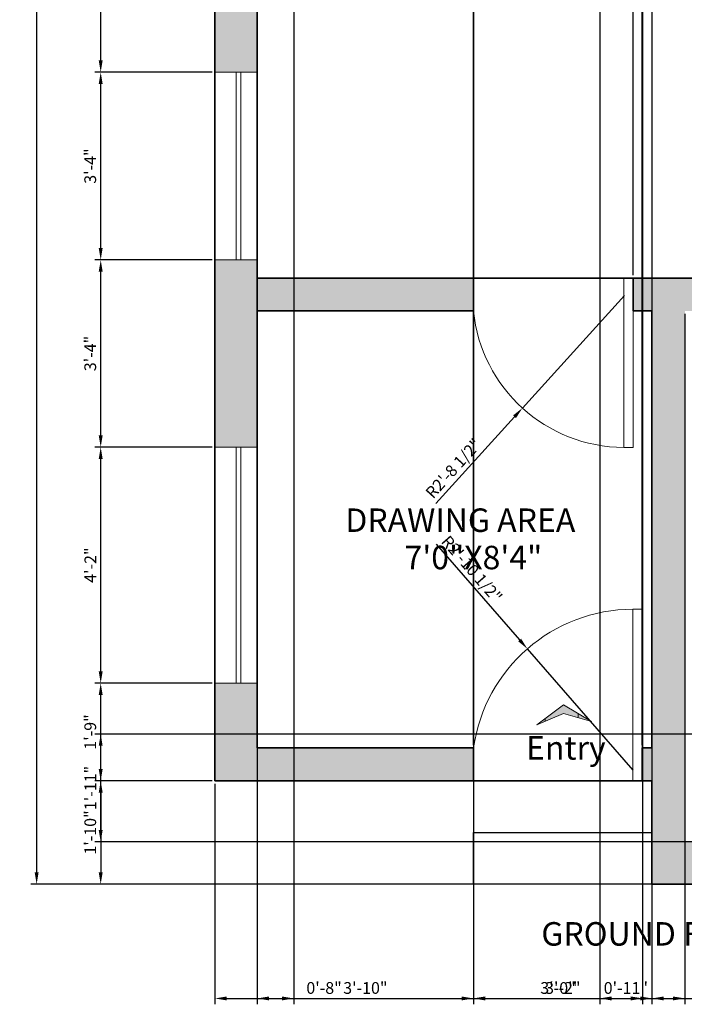
# Model space of a CAD drawing. Units: millimetres. Extents: x 2466 to 2817, y 2000 to 2512.
# Tile 1 of 4: x 2466 to 2607, y 2001 to 2210. Entities that reach past the tile are written whole.
import ezdxf

# ---------------------------------------------------------------- set-up
doc = ezdxf.new("R2010")
doc.units = ezdxf.units.MM
for name, color, linetype, lineweight in [('A-ANNO-DIMS', 2, 'Continuous', 13), ('A-ANNO-PATT', 7, 'Continuous', 13), ('A-ANNO-SYMB', 1, 'Continuous', 18), ('A-ANNO-TEXT', 7, 'Continuous', 18), ('A-AREA-IDEN', 7, 'Continuous', 18), ('A-DOOR', 3, 'Continuous', 18), ('A-FLOR-STRS', 7, 'Continuous', 25), ('A-GLAZ', 5, 'Continuous', 18), ('A-WALL', 7, 'Continuous', 35), ('A-WALL-PATT', 8, 'Continuous', 13)]:
    doc.layers.add(name, color=color, linetype=linetype, lineweight=lineweight)
doc.styles.get("Standard").update_dxf_attribs({"font": 'arial.ttf'})
doc.dimstyles.new('ISO-25', dxfattribs={"dimtxt": 2.5, "dimasz": 2.5, "dimexe": 1.25, "dimexo": 0.625, "dimtad": 1, "dimdec": 0, "dimlunit": 3, "dimtxsty": 'Standard', "dimcen": 2.5, "dimadec": 0, "dimazin": 0, "dimtfac": 1, "dimtdec": 0, "dimtmove": 0, "dimatfit": 3, "dimfxl": 1, "dimarcsym": 0})

# ---------------------------------------------------------------- blocks, each defined once
blk = doc.blocks.new('*D10')
at = {"layer": 'A-ANNO-DIMS', "color": 0, "lineweight": -2, "transparency": 16777216}
for p, q in [((2746.56, 2482.15), (2467.98, 2482.15)), ((2469.23, 2479.65), (2469.23, 2028.65)), ((2746.56, 2026.15), (2467.98, 2026.15))]:
    blk.add_line(p, q, dxfattribs=at)
at = {"layer": 'A-ANNO-DIMS', "color": 0, "transparency": 16777216}
for points in [[(2468.82, 2479.65), (2469.65, 2479.65), (2469.23, 2482.15)], [(2468.82, 2028.65), (2469.65, 2028.65), (2469.23, 2026.15)]]:
    blk.add_solid(points, dxfattribs=at)
at = {"layer": 'Defpoints', "color": 0, "transparency": 16777216}
for p in [(2747.19, 2482.15), (2469.23, 2026.15), (2747.19, 2026.15)]:
    blk.add_point(p, dxfattribs=at)
at = {"layer": 'A-ANNO-DIMS', "color": 0, "transparency": 16777216, "insert": (2467.33, 2254.15), "char_height": 2.5, "attachment_point": 5, "rotation": 90}
blk.add_mtext("38'", dxfattribs=at)
blk = doc.blocks.new('*D26')
at = {"layer": 'A-ANNO-DIMS', "color": 0, "lineweight": -2, "transparency": 16777216}
for p, q in [((2791.19, 2202.52), (2791.19, 2000.58)), ((2507.19, 2047.52), (2507.19, 2000.58)), ((2509.69, 2001.83), (2788.69, 2001.83))]:
    blk.add_line(p, q, dxfattribs=at)
at = {"layer": 'A-ANNO-DIMS', "color": 0, "transparency": 16777216}
for points in [[(2509.69, 2002.24), (2509.69, 2001.41), (2507.19, 2001.83)], [(2788.69, 2002.24), (2788.69, 2001.41), (2791.19, 2001.83)]]:
    blk.add_solid(points, dxfattribs=at)
at = {"layer": 'Defpoints', "color": 0, "transparency": 16777216}
for p in [(2791.19, 2203.15), (2507.19, 2048.15), (2791.19, 2001.83)]:
    blk.add_point(p, dxfattribs=at)
at = {"layer": 'A-ANNO-DIMS', "color": 0, "transparency": 16777216, "insert": (2649.19, 2003.73), "char_height": 2.5, "attachment_point": 5}
blk.add_mtext('23\'-8"', dxfattribs=at)
blk = doc.blocks.new('*D27')
at = {"layer": 'A-ANNO-DIMS', "color": 0, "lineweight": -2, "transparency": 16777216}
for p, q in [((2506.56, 2068.93), (2481.62, 2068.93)), ((2482.87, 2050.65), (2482.87, 2066.43)), ((2506.56, 2048.15), (2481.62, 2048.15))]:
    blk.add_line(p, q, dxfattribs=at)
at = {"layer": 'A-ANNO-DIMS', "color": 0, "transparency": 16777216}
for points in [[(2482.45, 2066.43), (2483.28, 2066.43), (2482.87, 2068.93)], [(2482.45, 2050.65), (2483.28, 2050.65), (2482.87, 2048.15)]]:
    blk.add_solid(points, dxfattribs=at)
at = {"layer": 'Defpoints', "color": 0, "transparency": 16777216}
for p in [(2482.87, 2068.93), (2507.19, 2068.93), (2507.19, 2048.15)]:
    blk.add_point(p, dxfattribs=at)
at = {"layer": 'A-ANNO-DIMS', "color": 0, "transparency": 16777216, "insert": (2480.97, 2058.54), "char_height": 2.5, "attachment_point": 5, "rotation": 90}
blk.add_mtext('1\'-9"', dxfattribs=at)
blk = doc.blocks.new('*D28')
at = {"layer": 'A-ANNO-DIMS', "color": 0, "lineweight": -2, "transparency": 16777216}
for p, q in [((2506.56, 2119.17), (2481.62, 2119.17)), ((2482.87, 2071.43), (2482.87, 2116.67)), ((2506.56, 2068.93), (2481.62, 2068.93))]:
    blk.add_line(p, q, dxfattribs=at)
at = {"layer": 'A-ANNO-DIMS', "color": 0, "transparency": 16777216}
for points in [[(2482.45, 2116.67), (2483.28, 2116.67), (2482.87, 2119.17)], [(2482.45, 2071.43), (2483.28, 2071.43), (2482.87, 2068.93)]]:
    blk.add_solid(points, dxfattribs=at)
at = {"layer": 'Defpoints', "color": 0, "transparency": 16777216}
for p in [(2482.87, 2119.17), (2507.19, 2119.17), (2507.19, 2068.93)]:
    blk.add_point(p, dxfattribs=at)
at = {"layer": 'A-ANNO-DIMS', "color": 0, "transparency": 16777216, "insert": (2480.99, 2094.05), "char_height": 2.5, "attachment_point": 5, "rotation": 90}
blk.add_mtext('4\'-2"', dxfattribs=at)
blk = doc.blocks.new('*D29')
at = {"layer": 'A-ANNO-DIMS', "color": 0, "lineweight": -2, "transparency": 16777216}
for p, q in [((2506.56, 2159.02), (2481.62, 2159.02)), ((2482.87, 2121.67), (2482.87, 2156.52)), ((2506.56, 2119.17), (2481.62, 2119.17))]:
    blk.add_line(p, q, dxfattribs=at)
at = {"layer": 'A-ANNO-DIMS', "color": 0, "transparency": 16777216}
for points in [[(2482.45, 2156.52), (2483.28, 2156.52), (2482.87, 2159.02)], [(2482.45, 2121.67), (2483.28, 2121.67), (2482.87, 2119.17)]]:
    blk.add_solid(points, dxfattribs=at)
at = {"layer": 'Defpoints', "color": 0, "transparency": 16777216}
for p in [(2482.87, 2159.02), (2507.19, 2159.02), (2507.19, 2119.17)]:
    blk.add_point(p, dxfattribs=at)
at = {"layer": 'A-ANNO-DIMS', "color": 0, "transparency": 16777216, "insert": (2480.96, 2139.1), "char_height": 2.5, "attachment_point": 5, "rotation": 90}
blk.add_mtext('3\'-4"', dxfattribs=at)
blk = doc.blocks.new('*D30')
at = {"layer": 'A-ANNO-DIMS', "color": 0, "lineweight": -2, "transparency": 16777216}
for p, q in [((2506.56, 2198.97), (2481.62, 2198.97)), ((2482.87, 2161.52), (2482.87, 2196.47)), ((2506.56, 2159.02), (2481.62, 2159.02))]:
    blk.add_line(p, q, dxfattribs=at)
at = {"layer": 'A-ANNO-DIMS', "color": 0, "transparency": 16777216}
for points in [[(2482.45, 2196.47), (2483.28, 2196.47), (2482.87, 2198.97)], [(2482.45, 2161.52), (2483.28, 2161.52), (2482.87, 2159.02)]]:
    blk.add_solid(points, dxfattribs=at)
at = {"layer": 'Defpoints', "color": 0, "transparency": 16777216}
for p in [(2482.87, 2198.97), (2507.19, 2198.97), (2507.19, 2159.02)]:
    blk.add_point(p, dxfattribs=at)
at = {"layer": 'A-ANNO-DIMS', "color": 0, "transparency": 16777216, "insert": (2480.96, 2178.99), "char_height": 2.5, "attachment_point": 5, "rotation": 90}
blk.add_mtext('3\'-4"', dxfattribs=at)
blk = doc.blocks.new('*D31')
at = {"layer": 'A-ANNO-DIMS', "color": 0, "lineweight": -2, "transparency": 16777216}
for p, q in [((2506.56, 2264.15), (2481.62, 2264.15)), ((2482.87, 2201.47), (2482.87, 2261.65)), ((2506.56, 2198.97), (2481.62, 2198.97))]:
    blk.add_line(p, q, dxfattribs=at)
at = {"layer": 'A-ANNO-DIMS', "color": 0, "transparency": 16777216}
for points in [[(2482.45, 2261.65), (2483.28, 2261.65), (2482.87, 2264.15)], [(2482.45, 2201.47), (2483.28, 2201.47), (2482.87, 2198.97)]]:
    blk.add_solid(points, dxfattribs=at)
at = {"layer": 'Defpoints', "color": 0, "transparency": 16777216}
for p in [(2482.87, 2264.15), (2507.19, 2264.15), (2507.19, 2198.97)]:
    blk.add_point(p, dxfattribs=at)
at = {"layer": 'A-ANNO-DIMS', "color": 0, "transparency": 16777216, "insert": (2480.97, 2231.56), "char_height": 2.5, "attachment_point": 5, "rotation": 90}
blk.add_mtext('5\'-5"', dxfattribs=at)
blk = doc.blocks.new('*D40')
at = {"layer": 'A-ANNO-DIMS', "color": 0, "lineweight": -2, "transparency": 16777216}
for p, q in [((2589.08, 2472.52), (2589.08, 2000.58)), ((2600.19, 2472.52), (2600.19, 2000.58)), ((2591.58, 2001.83), (2597.69, 2001.83))]:
    blk.add_line(p, q, dxfattribs=at)
at = {"layer": 'A-ANNO-DIMS', "color": 0, "transparency": 16777216}
for points in [[(2591.58, 2002.24), (2591.58, 2001.41), (2589.08, 2001.83)], [(2597.69, 2002.24), (2597.69, 2001.41), (2600.19, 2001.83)]]:
    blk.add_solid(points, dxfattribs=at)
at = {"layer": 'Defpoints', "color": 0, "transparency": 16777216}
for p in [(2589.08, 2473.15), (2600.19, 2473.15), (2600.19, 2001.83)]:
    blk.add_point(p, dxfattribs=at)
at = {"layer": 'A-ANNO-DIMS', "color": 0, "transparency": 16777216, "insert": (2594.63, 2003.73), "char_height": 2.5, "attachment_point": 5}
blk.add_mtext('0\'-11"', dxfattribs=at)
blk = doc.blocks.new('*D44')
at = {"layer": 'A-ANNO-DIMS', "color": 0, "lineweight": -2, "transparency": 16777216}
for p, q in [((2516.19, 2055.77), (2516.19, 2507.72)), ((2518.69, 2506.47), (2559.74, 2506.47)), ((2562.24, 2055.77), (2562.24, 2507.72))]:
    blk.add_line(p, q, dxfattribs=at)
at = {"layer": 'A-ANNO-DIMS', "color": 0, "transparency": 16777216}
for points in [[(2518.69, 2506.88), (2518.69, 2506.05), (2516.19, 2506.47)], [(2559.74, 2506.88), (2559.74, 2506.05), (2562.24, 2506.47)]]:
    blk.add_solid(points, dxfattribs=at)
at = {"layer": 'Defpoints', "color": 0, "transparency": 16777216}
for p in [(2562.24, 2506.47), (2516.19, 2055.15), (2562.24, 2055.15)]:
    blk.add_point(p, dxfattribs=at)
at = {"layer": 'A-ANNO-DIMS', "color": 0, "transparency": 16777216, "insert": (2539.21, 2508.37), "char_height": 2.5, "attachment_point": 5}
blk.add_mtext('3\'-10"', dxfattribs=at)
blk = doc.blocks.new('*D45')
at = {"layer": 'A-ANNO-DIMS', "color": 0, "lineweight": -2, "transparency": 16777216}
for p, q in [((2562.24, 2047.52), (2562.24, 2000.58)), ((2600.19, 2047.52), (2600.19, 2000.58)), ((2564.74, 2001.83), (2597.69, 2001.83))]:
    blk.add_line(p, q, dxfattribs=at)
at = {"layer": 'A-ANNO-DIMS', "color": 0, "transparency": 16777216}
for points in [[(2564.74, 2002.24), (2564.74, 2001.41), (2562.24, 2001.83)], [(2597.69, 2002.24), (2597.69, 2001.41), (2600.19, 2001.83)]]:
    blk.add_solid(points, dxfattribs=at)
at = {"layer": 'Defpoints', "color": 0, "transparency": 16777216}
for p in [(2562.24, 2048.15), (2600.19, 2048.15), (2600.19, 2001.83)]:
    blk.add_point(p, dxfattribs=at)
at = {"layer": 'A-ANNO-DIMS', "color": 0, "transparency": 16777216, "insert": (2581.21, 2003.73), "char_height": 2.5, "attachment_point": 5}
blk.add_mtext('3\'-2"', dxfattribs=at)
blk = doc.blocks.new('*D46')
at = {"layer": 'A-ANNO-DIMS', "color": 0, "lineweight": -2, "transparency": 16777216}
for p, q in [((2506.56, 2048.15), (2481.62, 2048.15)), ((2482.87, 2045.65), (2482.87, 2028.65)), ((2561.62, 2026.15), (2481.62, 2026.15))]:
    blk.add_line(p, q, dxfattribs=at)
at = {"layer": 'A-ANNO-DIMS', "color": 0, "transparency": 16777216}
for points in [[(2482.45, 2045.65), (2483.28, 2045.65), (2482.87, 2048.15)], [(2482.45, 2028.65), (2483.28, 2028.65), (2482.87, 2026.15)]]:
    blk.add_solid(points, dxfattribs=at)
at = {"layer": 'Defpoints', "color": 0, "transparency": 16777216}
for p in [(2507.19, 2048.15), (2482.87, 2026.15), (2562.24, 2026.15)]:
    blk.add_point(p, dxfattribs=at)
at = {"layer": 'A-ANNO-DIMS', "color": 0, "transparency": 16777216, "insert": (2480.97, 2037.15), "char_height": 2.5, "attachment_point": 5, "rotation": 90}
blk.add_mtext('1\'-10"', dxfattribs=at)
blk = doc.blocks.new('*D47')
at = {"layer": 'A-ANNO-DIMS', "color": 0, "lineweight": -2, "transparency": 16777216}
for p, q in [((2516.19, 2348.52), (2516.19, 2000.58)), ((2562.19, 2348.52), (2562.19, 2000.58)), ((2518.69, 2001.83), (2559.69, 2001.83))]:
    blk.add_line(p, q, dxfattribs=at)
at = {"layer": 'A-ANNO-DIMS', "color": 0, "transparency": 16777216}
for points in [[(2518.69, 2002.24), (2518.69, 2001.41), (2516.19, 2001.83)], [(2559.69, 2002.24), (2559.69, 2001.41), (2562.19, 2001.83)]]:
    blk.add_solid(points, dxfattribs=at)
at = {"layer": 'Defpoints', "color": 0, "transparency": 16777216}
for p in [(2516.19, 2349.15), (2562.19, 2349.15), (2562.19, 2001.83)]:
    blk.add_point(p, dxfattribs=at)
at = {"layer": 'A-ANNO-DIMS', "color": 0, "transparency": 16777216, "insert": (2539.19, 2003.73), "char_height": 2.5, "attachment_point": 5}
blk.add_mtext('3\'-10"', dxfattribs=at)
blk = doc.blocks.new('*D48')
at = {"layer": 'A-ANNO-DIMS', "color": 0, "lineweight": -2, "transparency": 16777216}
for p, q in [((2562.19, 2348.52), (2562.19, 2000.58)), ((2598.19, 2348.52), (2598.19, 2000.58)), ((2564.69, 2001.83), (2595.69, 2001.83))]:
    blk.add_line(p, q, dxfattribs=at)
at = {"layer": 'A-ANNO-DIMS', "color": 0, "transparency": 16777216}
for points in [[(2564.69, 2002.24), (2564.69, 2001.41), (2562.19, 2001.83)], [(2595.69, 2002.24), (2595.69, 2001.41), (2598.19, 2001.83)]]:
    blk.add_solid(points, dxfattribs=at)
at = {"layer": 'Defpoints', "color": 0, "transparency": 16777216}
for p in [(2562.19, 2349.15), (2598.19, 2349.15), (2598.19, 2001.83)]:
    blk.add_point(p, dxfattribs=at)
at = {"layer": 'A-ANNO-DIMS', "color": 0, "transparency": 16777216, "insert": (2580.19, 2003.73), "char_height": 2.5, "attachment_point": 5}
blk.add_mtext('3\'-0"', dxfattribs=at)
blk = doc.blocks.new('*D51')
at = {"layer": 'A-ANNO-DIMS', "color": 0, "lineweight": -2, "transparency": 16777216}
for p, q in [((2516.19, 2155.77), (2516.19, 2507.72)), ((2518.69, 2506.47), (2559.69, 2506.47)), ((2562.19, 2155.77), (2562.19, 2507.72))]:
    blk.add_line(p, q, dxfattribs=at)
at = {"layer": 'A-ANNO-DIMS', "color": 0, "transparency": 16777216}
for points in [[(2518.69, 2506.88), (2518.69, 2506.05), (2516.19, 2506.47)], [(2559.69, 2506.88), (2559.69, 2506.05), (2562.19, 2506.47)]]:
    blk.add_solid(points, dxfattribs=at)
at = {"layer": 'Defpoints', "color": 0, "transparency": 16777216}
for p in [(2562.19, 2506.47), (2516.19, 2155.15), (2562.19, 2155.15)]:
    blk.add_point(p, dxfattribs=at)
at = {"layer": 'A-ANNO-DIMS', "color": 0, "transparency": 16777216, "insert": (2539.19, 2508.37), "char_height": 2.5, "attachment_point": 5}
blk.add_mtext('3\'-10"', dxfattribs=at)
blk = doc.blocks.new('*D52')
at = {"layer": 'A-ANNO-DIMS', "color": 0, "lineweight": -2, "transparency": 16777216}
for p, q in [((2562.19, 2155.77), (2562.19, 2507.72)), ((2564.69, 2506.47), (2593.69, 2506.47)), ((2596.19, 2155.77), (2596.19, 2507.72))]:
    blk.add_line(p, q, dxfattribs=at)
at = {"layer": 'A-ANNO-DIMS', "color": 0, "transparency": 16777216}
for points in [[(2564.69, 2506.88), (2564.69, 2506.05), (2562.19, 2506.47)], [(2593.69, 2506.88), (2593.69, 2506.05), (2596.19, 2506.47)]]:
    blk.add_solid(points, dxfattribs=at)
at = {"layer": 'Defpoints', "color": 0, "transparency": 16777216}
for p in [(2596.19, 2506.47), (2562.19, 2155.15), (2596.19, 2155.15)]:
    blk.add_point(p, dxfattribs=at)
at = {"layer": 'A-ANNO-DIMS', "color": 0, "transparency": 16777216, "insert": (2579.19, 2508.37), "char_height": 2.5, "attachment_point": 5}
blk.add_mtext('2\'-10"', dxfattribs=at)
blk = doc.blocks.new('*D53')
at = {"layer": 'A-ANNO-DIMS', "color": 0, "lineweight": -2, "transparency": 16777216}
for p, q in [((2596.19, 2155.77), (2596.19, 2507.72)), ((2598.69, 2506.47), (2608.69, 2506.47)), ((2611.19, 2155.77), (2611.19, 2507.72))]:
    blk.add_line(p, q, dxfattribs=at)
at = {"layer": 'A-ANNO-DIMS', "color": 0, "transparency": 16777216}
for points in [[(2598.69, 2506.88), (2598.69, 2506.05), (2596.19, 2506.47)], [(2608.69, 2506.88), (2608.69, 2506.05), (2611.19, 2506.47)]]:
    blk.add_solid(points, dxfattribs=at)
at = {"layer": 'Defpoints', "color": 0, "transparency": 16777216}
for p in [(2611.19, 2506.47), (2596.19, 2155.15), (2611.19, 2155.15)]:
    blk.add_point(p, dxfattribs=at)
at = {"layer": 'A-ANNO-DIMS', "color": 0, "transparency": 16777216, "insert": (2603.69, 2508.37), "char_height": 2.5, "attachment_point": 5}
blk.add_mtext('1\'-3"', dxfattribs=at)
blk = doc.blocks.new('*D59')
at = {"layer": 'A-ANNO-DIMS', "color": 0, "lineweight": -2, "transparency": 16777216}
for p, q in [((2600.19, 2147.52), (2600.19, 2000.58)), ((2607.19, 2147.52), (2607.19, 2000.58)), ((2602.69, 2001.83), (2604.69, 2001.83)), ((2607.19, 2001.83), (2617.58, 2001.83))]:
    blk.add_line(p, q, dxfattribs=at)
at = {"layer": 'A-ANNO-DIMS', "color": 0, "transparency": 16777216}
for points in [[(2602.69, 2002.24), (2602.69, 2001.41), (2600.19, 2001.83)], [(2604.69, 2002.24), (2604.69, 2001.41), (2607.19, 2001.83)]]:
    blk.add_solid(points, dxfattribs=at)
at = {"layer": 'Defpoints', "color": 0, "transparency": 16777216}
for p in [(2600.19, 2148.15), (2607.19, 2148.15), (2607.19, 2001.83)]:
    blk.add_point(p, dxfattribs=at)
at = {"layer": 'A-ANNO-DIMS', "color": 0, "transparency": 16777216, "insert": (2613.63, 2003.73), "char_height": 2.5, "attachment_point": 5}
blk.add_mtext('0\'-7"', dxfattribs=at)
blk = doc.blocks.new('*D64')
at = {"layer": 'A-ANNO-DIMS', "color": 0, "lineweight": -2, "transparency": 16777216}
for p, q in [((2562.24, 2055.77), (2562.24, 2507.72)), ((2564.74, 2506.47), (2595.62, 2506.47)), ((2598.12, 2055.77), (2598.12, 2507.72))]:
    blk.add_line(p, q, dxfattribs=at)
at = {"layer": 'A-ANNO-DIMS', "color": 0, "transparency": 16777216}
for points in [[(2564.74, 2506.88), (2564.74, 2506.05), (2562.24, 2506.47)], [(2595.62, 2506.88), (2595.62, 2506.05), (2598.12, 2506.47)]]:
    blk.add_solid(points, dxfattribs=at)
at = {"layer": 'Defpoints', "color": 0, "transparency": 16777216}
for p in [(2598.12, 2506.47), (2562.24, 2055.15), (2598.12, 2055.15)]:
    blk.add_point(p, dxfattribs=at)
at = {"layer": 'A-ANNO-DIMS', "color": 0, "transparency": 16777216, "insert": (2580.18, 2508.37), "char_height": 2.5, "attachment_point": 5}
blk.add_mtext('3\'-0"', dxfattribs=at)
blk = doc.blocks.new('*D68')
at = {"layer": 'A-ANNO-DIMS', "color": 0, "lineweight": -2, "transparency": 16777216}
for p, q in [((2737.56, 2058.1), (2481.62, 2058.1)), ((2482.87, 2037.65), (2482.87, 2055.6)), ((2737.56, 2035.15), (2481.62, 2035.15))]:
    blk.add_line(p, q, dxfattribs=at)
at = {"layer": 'A-ANNO-DIMS', "color": 0, "transparency": 16777216}
for points in [[(2482.45, 2055.6), (2483.28, 2055.6), (2482.87, 2058.1)], [(2482.45, 2037.65), (2483.28, 2037.65), (2482.87, 2035.15)]]:
    blk.add_solid(points, dxfattribs=at)
at = {"layer": 'Defpoints', "color": 0, "transparency": 16777216}
for p in [(2482.87, 2058.1), (2738.19, 2058.1), (2738.19, 2035.15)]:
    blk.add_point(p, dxfattribs=at)
at = {"layer": 'A-ANNO-DIMS', "color": 0, "transparency": 16777216, "insert": (2480.99, 2046.62), "char_height": 2.5, "attachment_point": 5, "rotation": 90}
blk.add_mtext('1\'-11"', dxfattribs=at)
blk = doc.blocks.new('*D71')
at = {"layer": 'A-ANNO-DIMS', "color": 0, "lineweight": -2, "transparency": 16777216}
for p, q in [((2523.95, 2389.93), (2523.95, 2000.58)), ((2516.19, 2383.21), (2516.19, 2000.58)), ((2518.69, 2001.83), (2521.45, 2001.83)), ((2523.95, 2001.83), (2534.35, 2001.83))]:
    blk.add_line(p, q, dxfattribs=at)
at = {"layer": 'A-ANNO-DIMS', "color": 0, "transparency": 16777216}
for points in [[(2518.69, 2002.24), (2518.69, 2001.41), (2516.19, 2001.83)], [(2521.45, 2002.24), (2521.45, 2001.41), (2523.95, 2001.83)]]:
    blk.add_solid(points, dxfattribs=at)
at = {"layer": 'Defpoints', "color": 0, "transparency": 16777216}
for p in [(2523.95, 2390.56), (2516.19, 2383.84), (2523.95, 2001.83)]:
    blk.add_point(p, dxfattribs=at)
at = {"layer": 'A-ANNO-DIMS', "color": 0, "transparency": 16777216, "insert": (2530.4, 2003.73), "char_height": 2.5, "attachment_point": 5}
blk.add_mtext('0\'-8"', dxfattribs=at)
blk = doc.blocks.new('*D77')
at = {"layer": 'A-ANNO-DIMS', "color": 0, "lineweight": -2, "transparency": 16777216}
for p, q in [((2554.24, 2098.54), (2572.03, 2078.12)), ((2596.17, 2050.41), (2573.67, 2076.24))]:
    blk.add_line(p, q, dxfattribs=at)
at = {"layer": 'A-ANNO-DIMS', "color": 0, "transparency": 16777216}
blk.add_solid([(2572.34, 2078.4), (2571.71, 2077.85), (2573.67, 2076.24)], dxfattribs=at)
at = {"layer": 'Defpoints', "color": 0, "transparency": 16777216}
for p in [(2573.67, 2076.24), (2596.17, 2050.41)]:
    blk.add_point(p, dxfattribs=at)
at = {"layer": 'A-ANNO-DIMS', "color": 0, "transparency": 16777216, "insert": (2561.61, 2093), "char_height": 2.5, "attachment_point": 5, "rotation": 311.0599}
blk.add_mtext('R2\'-10 1/2"', dxfattribs=at)
blk = doc.blocks.new('*D78')
at = {"layer": 'A-ANNO-DIMS', "color": 0, "lineweight": -2, "transparency": 16777216}
for p, q in [((2594.35, 2151.42), (2572.62, 2127.49)), ((2554.16, 2107.16), (2570.94, 2125.64))]:
    blk.add_line(p, q, dxfattribs=at)
at = {"layer": 'A-ANNO-DIMS', "color": 0, "transparency": 16777216}
blk.add_solid([(2570.63, 2125.92), (2571.25, 2125.36), (2572.62, 2127.49)], dxfattribs=at)
at = {"layer": 'Defpoints', "color": 0, "transparency": 16777216}
for p in [(2594.35, 2151.42), (2572.62, 2127.49)]:
    blk.add_point(p, dxfattribs=at)
at = {"layer": 'A-ANNO-DIMS', "color": 0, "transparency": 16777216, "insert": (2558.16, 2114.42), "char_height": 2.5, "attachment_point": 5, "rotation": 47.7645}
blk.add_mtext('R2\'-8 1/2"', dxfattribs=at)

msp = doc.modelspace()

# ---------------------------------------------------------------- hatches: boundary and pattern name
at = {"layer": 'A-ANNO-PATT'}
h = msp.add_hatch(dxfattribs=at)
h.set_pattern_fill('ANGLE', color=256)
h.set_pattern_definition([(0, (0, 0), (0, 6.985), [5.08, -1.905]), (90, (0, 0), (-6.985, 4e-16), [5.08, -1.905])])
h.paths.add_polyline_path([(2581.33, 2064.29), (2575.65, 2060.04), (2581.38, 2062.44), (2587.31, 2060.79)])
h = msp.add_hatch(color=256, dxfattribs=at)
h.dxf.hatch_style = 1
h.paths.add_polyline_path([(2581.33, 2064.29), (2575.65, 2060.04), (2581.38, 2062.44), (2587.31, 2060.79)])
at = {"layer": 'A-WALL-PATT'}
h = msp.add_hatch(color=256, dxfattribs=at)
h.dxf.hatch_style = 1
h.paths.add_polyline_path([(2516.19, 2264.15), (2507.19, 2264.15), (2507.19, 2198.97), (2516.19, 2198.97)])
h = msp.add_hatch(color=256, dxfattribs=at)
h.dxf.hatch_style = 1
h.paths.add_polyline_path([(2516.19, 2159.02), (2507.19, 2159.02), (2507.19, 2119.17), (2516.19, 2119.17)])
h.paths.add_polyline_path([(2516.19, 2068.93), (2507.19, 2068.93), (2507.19, 2048.15), (2516.19, 2048.15), (2562.24, 2048.15), (2562.24, 2055.15), (2551.24, 2055.15), (2516.19, 2055.15)])
h.paths.add_polyline_path([(2607.19, 2148.15), (2611.19, 2148.15), (2611.19, 2155.15), (2596.19, 2155.15), (2596.19, 2148.15), (2600.19, 2148.15), (2600.19, 2055.15), (2598.12, 2055.15), (2598.12, 2048.15), (2600.19, 2048.15), (2600.19, 2035.15), (2600.19, 2026.15), (2606.96, 2026.15), (2650.11, 2026.15), (2650.11, 2035.15), (2607.19, 2035.15)])
h = msp.add_hatch(color=256, dxfattribs=at)
h.dxf.hatch_style = 1
h.paths.add_polyline_path([(2562.19, 2155.15), (2516.19, 2155.15), (2516.19, 2148.15), (2562.19, 2148.15)])

# ---------------------------------------------------------------- linework, layer by layer
at = {"layer": 'A-ANNO-SYMB'}
msp.add_lwpolyline([(2575.65, 2060.04), (2581.38, 2062.44), (2587.31, 2060.79), (2581.33, 2064.29)], close=True, dxfattribs=at)
at = {"layer": 'A-DOOR'}
for p, q in [((2594.19, 2119.1), (2594.19, 2155.15)), ((2596.19, 2148.15), (2596.19, 2119.1)), ((2596.19, 2119.1), (2594.19, 2119.1)), ((2598.12, 2084.66), (2596.12, 2084.66)), ((2596.12, 2084.66), (2596.12, 2048.15)), ((2598.12, 2055.15), (2598.12, 2084.66))]:
    msp.add_line(p, q, dxfattribs=at)
for centre, radius, start, end in [((2594.35, 2151.42), 32.32, 185.8104, 269.7186), ((2596.17, 2050.41), 34.26, 90.0766, 172.0433)]:
    msp.add_arc(centre, radius, start, end, dxfattribs=at)
at = {"layer": 'A-FLOR-STRS'}
for p, q in [((2562.24, 2048.15), (2562.24, 2037.15)), ((2562.24, 2037.15), (2600.19, 2037.15)), ((2562.24, 2026.15), (2562.24, 2037.15)), ((2600.19, 2037.15), (2600.19, 2026.15)), ((2600.19, 2026.15), (2562.24, 2026.15))]:
    msp.add_line(p, q, dxfattribs=at)
at = {"layer": 'A-GLAZ'}
for p, q in [((2516.19, 2198.97), (2507.19, 2198.97)), ((2507.19, 2198.97), (2507.19, 2159.02)), ((2511.69, 2198.97), (2511.69, 2159.02)), ((2512.69, 2198.97), (2512.69, 2159.02)), ((2516.19, 2159.02), (2516.19, 2198.97)), ((2507.19, 2159.02), (2516.19, 2159.02)), ((2507.19, 2119.17), (2516.19, 2119.17)), ((2507.19, 2068.93), (2507.19, 2119.17)), ((2511.69, 2119.17), (2511.69, 2068.93)), ((2512.69, 2119.17), (2512.69, 2068.93)), ((2516.19, 2119.17), (2516.19, 2068.93)), ((2516.19, 2068.93), (2507.19, 2068.93))]:
    msp.add_line(p, q, dxfattribs=at)
at = {"layer": 'A-WALL'}
for p, q in [((2507.19, 2048.15), (2507.19, 2482.15)), ((2516.19, 2055.15), (2516.19, 2473.15)), ((2642.19, 2155.15), (2516.19, 2155.15)), ((2562.19, 2155.15), (2562.19, 2148.15)), ((2596.19, 2148.15), (2596.19, 2155.15)), ((2562.19, 2148.15), (2516.19, 2148.15)), ((2600.19, 2148.15), (2596.19, 2148.15)), ((2600.19, 2055.15), (2600.19, 2148.15)), ((2551.24, 2055.15), (2516.19, 2055.15)), ((2551.24, 2055.15), (2562.24, 2055.15)), ((2562.24, 2055.15), (2562.24, 2048.15)), ((2600.19, 2055.15), (2598.12, 2055.15)), ((2598.12, 2055.15), (2598.12, 2048.15)), ((2516.19, 2048.15), (2507.19, 2048.15)), ((2600.19, 2048.15), (2516.19, 2048.15)), ((2562.24, 2048.15), (2562.24, 2048.15)), ((2600.19, 2035.15), (2600.19, 2048.15)), ((2600.19, 2035.15), (2600.19, 2026.15)), ((2600.19, 2026.15), (2600.19, 2026.15)), ((2606.96, 2026.15), (2600.19, 2026.15)), ((2747.19, 2026.15), (2606.96, 2026.15))]:
    msp.add_line(p, q, dxfattribs=at)

# ---------------------------------------------------------------- texts
at = {"layer": 'A-ANNO-TEXT'}
for s, p in [('Entry', (2573.39, 2052.66)), ('GROUND FLOOR PLAN', (2576.64, 2013.07))]:
    msp.add_text(s, height=5, dxfattribs=at).set_placement(p)
at = {"layer": 'A-AREA-IDEN'}
for s, p in [('DRAWING AREA', (2534.92, 2101.12)), ('7\'0"X8\'4"', (2547.53, 2093.17))]:
    msp.add_text(s, height=5, dxfattribs=at).set_placement(p)

# ---------------------------------------------------------------- dimensions: what is measured, and where the dimension line sits
at = {"layer": 'A-ANNO-DIMS'}
for base, p1, p2, picture, middle in [((2562.2416, 2506.4679), (2516.1868, 2055.1479), (2562.2416, 2055.1479), '*D44', (2539.2142, 2508.3702)), ((2562.19, 2506.47), (2516.19, 2155.15), (2562.19, 2155.15), '*D51', (2539.19, 2508.37)), ((2596.19, 2506.47), (2562.19, 2155.15), (2596.19, 2155.15), '*D52', (2579.19, 2508.37)), ((2598.12, 2506.47), (2562.24, 2055.15), (2598.12, 2055.15), '*D64', (2580.18, 2508.37)), ((2611.19, 2506.47), (2596.19, 2155.15), (2611.19, 2155.15), '*D53', (2603.69, 2508.37)), ((2600.19, 2001.83), (2589.08, 2473.15), (2600.19, 2473.15), '*D40', (2594.63, 2003.73)), ((2523.95, 2001.83), (2516.19, 2383.84), (2523.95, 2390.56), '*D71', (2530.4, 2003.73)), ((2562.19, 2001.83), (2516.19, 2349.15), (2562.19, 2349.15), '*D47', (2539.19, 2003.73)), ((2598.19, 2001.83), (2562.19, 2349.15), (2598.19, 2349.15), '*D48', (2580.19, 2003.73)), ((2791.19, 2001.83), (2507.19, 2048.15), (2791.19, 2203.15), '*D26', (2649.19, 2003.73)), ((2607.19, 2001.83), (2600.19, 2148.15), (2607.19, 2148.15), '*D59', (2613.63, 2003.73)), ((2600.1868, 2001.8279), (2562.2416, 2048.1479), (2600.1868, 2048.1479), '*D45', (2581.2142, 2003.7302))]:
    dim = msp.add_linear_dim(base=base, p1=p1, p2=p2, dimstyle='ISO-25', override={"dimdec": 1, "dimlfac": 1, "dimrnd": 0, "dimzin": 1, "dimdsep": 46, "dimlunit": 4, "dimfrac": 2}, dxfattribs=at)
    dim.commit()
    dim.dimension.update_dxf_attribs({"geometry": picture, "text_midpoint": middle})
for base, p1, p2, override, picture, middle in [((2469.23, 2026.15), (2747.19, 2482.15), (2747.19, 2026.15), {"dimclrd": 0, "dimclre": 0, "dimclrt": 0}, '*D10', (2467.33, 2254.15)), ((2482.87, 2264.15), (2507.19, 2198.97), (2507.19, 2264.15), {"dimdec": 1, "dimlfac": 1, "dimrnd": 0, "dimzin": 1, "dimdsep": 46, "dimlunit": 4, "dimfrac": 2}, '*D31', (2480.97, 2231.56)), ((2482.8668, 2198.9679), (2507.1868, 2159.0214), (2507.1868, 2198.9679), {"dimdec": 1, "dimlfac": 1, "dimrnd": 0, "dimzin": 1, "dimdsep": 46, "dimlunit": 4, "dimfrac": 2}, '*D30', (2480.9645, 2178.9947)), ((2482.8668, 2159.0214), (2507.1868, 2119.1745), (2507.1868, 2159.0214), {"dimdec": 1, "dimlfac": 1, "dimrnd": 0, "dimzin": 1, "dimdsep": 46, "dimlunit": 4, "dimfrac": 2}, '*D29', (2480.9645, 2139.098)), ((2482.87, 2119.17), (2507.19, 2068.93), (2507.19, 2119.17), {"dimdec": 1, "dimlfac": 1, "dimrnd": 0, "dimzin": 1, "dimdsep": 46, "dimlunit": 4, "dimfrac": 2}, '*D28', (2480.99, 2094.05)), ((2482.87, 2068.93), (2507.19, 2048.15), (2507.19, 2068.93), {"dimdec": 1, "dimlfac": 1, "dimrnd": 0, "dimzin": 1, "dimdsep": 46, "dimlunit": 4, "dimfrac": 2}, '*D27', (2480.97, 2058.54)), ((2482.8668, 2058.1003), (2738.1868, 2035.1479), (2738.1868, 2058.1003), {"dimdec": 1, "dimlfac": 1, "dimrnd": 0, "dimzin": 1, "dimdsep": 46, "dimlunit": 4, "dimfrac": 2}, '*D68', (2480.9867, 2046.6241)), ((2482.87, 2026.15), (2507.19, 2048.15), (2562.24, 2026.15), {"dimdec": 1, "dimlfac": 1, "dimrnd": 0, "dimzin": 1, "dimdsep": 46, "dimlunit": 4, "dimfrac": 2}, '*D46', (2480.97, 2037.15))]:
    dim = msp.add_linear_dim(base=base, p1=p1, p2=p2, angle=90, dimstyle='ISO-25', override=override, dxfattribs=at)
    dim.commit()
    dim.dimension.update_dxf_attribs({"geometry": picture, "text_midpoint": middle})
for center, mpoint, picture, middle in [((2594.35, 2151.42), (2572.62, 2127.49), '*D78', (2559.58, 2113.13)), ((2596.17, 2050.41), (2573.67, 2076.24), '*D77', (2560.17, 2091.74))]:
    dim = msp.add_radius_dim(center=center, mpoint=mpoint, dimstyle='ISO-25', override={"dimdec": 1, "dimlfac": 1, "dimrnd": 0, "dimzin": 1, "dimdsep": 46, "dimlunit": 4, "dimfrac": 2}, dxfattribs=at)
    dim.commit()
    dim.dimension.update_dxf_attribs({"geometry": picture, "text_midpoint": middle, "dimtype": 164})

doc.saveas('drawing.dxf')
